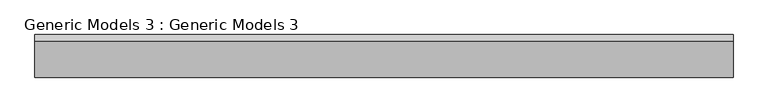
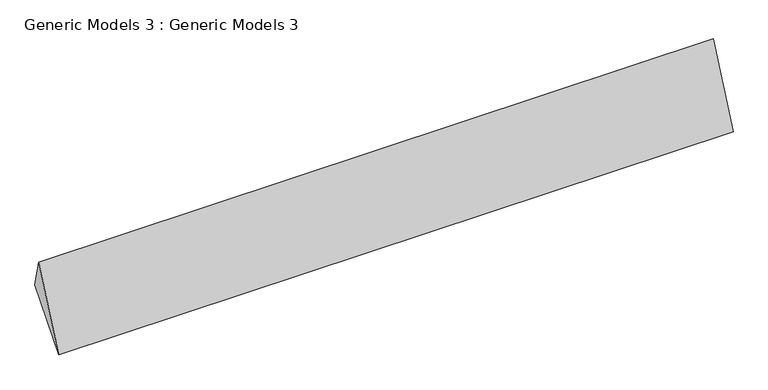
"""IFC4 building model written with IfcOpenShell, lengths in millimetres: proxy geometry, Generic Models 3 : Generic Models 3."""

from ifc_helpers import new_model, si_unit, frame, origin, place, context, project, spatial, polyline, outline, extrude, source, transform, mapped, element, save


def generic_models_3_generic_models_3_c0206aab(model_context):
    return source(origin(), model_context, "Body", "SweptSolid", [
        extrude(outline(polyline([(2174.8040133, -124.7280845), (2374.0227934, 322.7246217), (2413.2942675, 159.4935327), (2174.8040133, -124.7280845)])), frame((1731.970055, 0.0, 0.0), z_axis=(1.0, 0.0, 0.0), x_axis=(0.0, 1.0, 0.0)), (0.0, 0.0, 1.0), 3906.829945),
    ])


if __name__ == "__main__":
    model = new_model("IFC4")
    model_context = context("Model", 3, world=origin())
    ifc_project = project(units=[si_unit("LENGTHUNIT", "METRE", prefix="MILLI")], contexts=[model_context])
    site = spatial("IfcSite", under=ifc_project)
    building = spatial("IfcBuilding", under=site)
    placement = place(None, origin())
    generic_models_3_generic_models_3_shape = generic_models_3_generic_models_3_c0206aab(model_context)
    element("IfcBuildingElementProxy", 1, Name="Generic Models 3 : Generic Models 3", ObjectType="Generic Models 3 : Generic Models 3", at=placement, inside=building, context=model_context, shape_type="MappedRepresentation", body=[
        mapped(generic_models_3_generic_models_3_shape, transform((0.0, 0.0, 0.0), x_axis=(1.0, 0.0, 0.0), y_axis=(0.0, 1.0, 0.0), z_axis=(0.0, 0.0, 1.0))),
    ])
    save(model, "model.ifc")

# Revit data of these elements
# Element 1 (IfcBuildingElementProxy, "Generic Models 3 : Generic Models 3")
#   Materials on its faces: "Carpet (1)"
# Materials
#   "Carpet (1)": class "Carpet", colour RGB 124 80 67, transparency 0, Description = "Interior finish", Cost = 0
